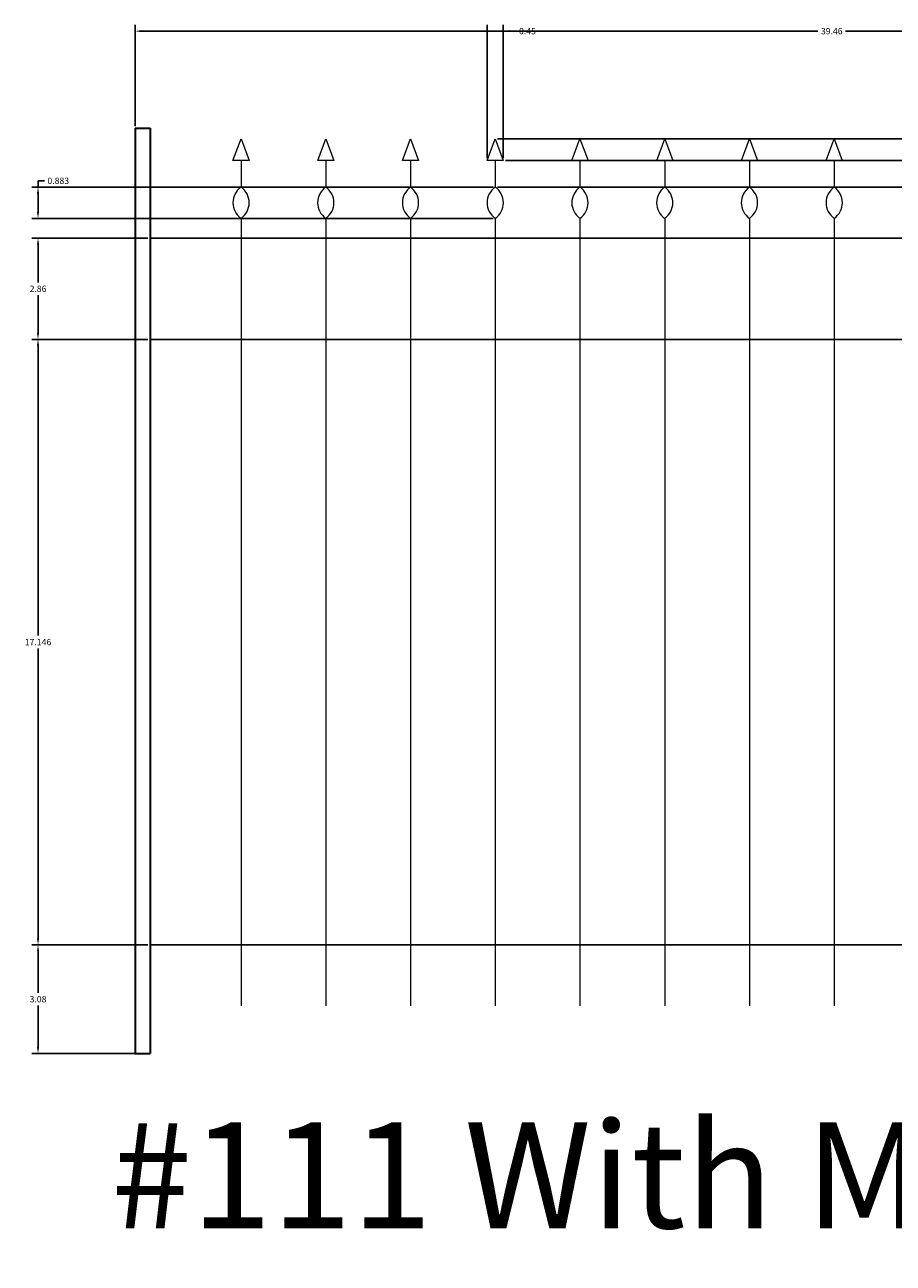
# Model space of a CAD drawing. Units: inches. Extents: x 756 to 915, y 488 to 695.
# Tile 24 of 25: x 863 to 888, y 660 to 695. Entities that reach past the tile are written whole.
import ezdxf

# ---------------------------------------------------------------- set-up
doc = ezdxf.new("R2010")
doc.units = ezdxf.units.IN
doc.header["$MEASUREMENT"] = 0
for name, color, linetype, lineweight in [('L-ANNO-TEXT', 7, 'Continuous', 25), ('L-FENC-PCKT', 7, 'Continuous', 18), ('L-FENC-POST', 7, 'Continuous', 35), ('L-FENC-RAIL', 7, 'Continuous', 25), ('M-DIMS', 2, 'Continuous', 18)]:
    doc.layers.add(name, color=color, linetype=linetype, lineweight=lineweight)
doc.styles.get("Standard").update_dxf_attribs({"font": 'arial.ttf'})
doc.dimstyles.get("Standard").update_dxf_attribs({"dimtxt": 0.18, "dimasz": 0.18, "dimexe": 0.18, "dimexo": 0.0625, "dimgap": 0.09, "dimtad": 0, "dimtih": 1, "dimtoh": 1, "dimdec": 0, "dimzin": 0, "dimdsep": 46, "dimlunit": 3, "dimtxsty": 'Standard', "dimcen": 0.09, "dimadec": 0, "dimazin": 0, "dimtfac": 1, "dimtdec": 0, "dimtofl": 0, "dimtmove": 0, "dimatfit": 3, "dimfxl": 1, "dimtolj": 1, "dimtzin": 0, "dimarcsym": 0})

# ---------------------------------------------------------------- blocks, each defined once
blk = doc.blocks.new('PICKET-MAJESTIC-EXTENDED')
for p, q in [((0.231, 23.946), (0.231, 23.188)), ((0.231, 22.305), (0.231, 0))]:
    blk.add_line(p, q)
blk.add_lwpolyline([(0.231, 23.946), (0.003, 23.946), (0.231, 24.558), (0.458, 23.946)], close=True)
blk.add_lwpolyline([(0.231, 22.305, 0.522719), (0.231, 23.188, 0.522719)], format="xyb", close=True)
blk = doc.blocks.new('FENCE-POST-LEFT')
for p, q in [((0, 26.207), (0, 0)), ((0, 26.207), (0.426, 26.207)), ((0.426, 26.207), (0.426, 0)), ((0.426, 26.207), (0.426, 0)), ((0, 0), (0.426, 0))]:
    blk.add_line(p, q)
blk = doc.blocks.new('*D23')
at = {"layer": 'Defpoints', "color": 0, "transparency": 16777216}
for p in [(905.684, 694.703), (866.226, 691.953), (905.684, 691.953)]:
    blk.add_point(p, dxfattribs=at)
at = {"layer": 'M-DIMS', "color": 0, "lineweight": -2, "transparency": 16777216}
for p, q in [((866.226, 692.015), (866.226, 694.883)), ((905.684, 692.015), (905.684, 694.883)), ((866.406, 694.703), (885.561, 694.703)), ((905.504, 694.703), (886.348, 694.703))]:
    blk.add_line(p, q, dxfattribs=at)
at = {"layer": 'M-DIMS', "color": 0, "transparency": 16777216}
for points in [[(866.406, 694.733), (866.406, 694.673), (866.226, 694.703)], [(905.504, 694.733), (905.504, 694.673), (905.684, 694.703)]]:
    blk.add_solid(points, dxfattribs=at)
at = {"layer": 'M-DIMS', "color": 0, "transparency": 16777216, "insert": (885.955, 694.703), "char_height": 0.18, "attachment_point": 5}
blk.add_mtext('\\A1;39.46', dxfattribs=at)
blk = doc.blocks.new('*D25')
at = {"layer": 'Defpoints', "color": 0, "transparency": 16777216}
for p in [(863.476, 685.974), (866.652, 685.974), (866.652, 668.828)]:
    blk.add_point(p, dxfattribs=at)
at = {"layer": 'M-DIMS', "color": 0, "lineweight": -2, "transparency": 16777216}
for p, q in [((866.59, 685.974), (863.296, 685.974)), ((863.476, 685.794), (863.476, 677.583)), ((863.476, 669.008), (863.476, 677.219)), ((866.59, 668.828), (863.296, 668.828))]:
    blk.add_line(p, q, dxfattribs=at)
at = {"layer": 'M-DIMS', "color": 0, "transparency": 16777216}
for points in [[(863.446, 685.794), (863.506, 685.794), (863.476, 685.974)], [(863.446, 669.008), (863.506, 669.008), (863.476, 668.828)]]:
    blk.add_solid(points, dxfattribs=at)
at = {"layer": 'M-DIMS', "color": 0, "transparency": 16777216, "insert": (863.476, 677.401), "char_height": 0.18, "attachment_point": 5}
blk.add_mtext('\\A1;17.146', dxfattribs=at)
blk = doc.blocks.new('*D26')
at = {"layer": 'Defpoints', "color": 0, "transparency": 16777216}
for p in [(863.476, 688.838), (866.652, 688.838), (866.652, 685.974)]:
    blk.add_point(p, dxfattribs=at)
at = {"layer": 'M-DIMS', "color": 0, "lineweight": -2, "transparency": 16777216}
for p, q in [((866.59, 688.838), (863.296, 688.838)), ((863.476, 688.658), (863.476, 687.588)), ((863.476, 686.154), (863.476, 687.224)), ((866.59, 685.974), (863.296, 685.974))]:
    blk.add_line(p, q, dxfattribs=at)
at = {"layer": 'M-DIMS', "color": 0, "transparency": 16777216}
for points in [[(863.446, 688.658), (863.506, 688.658), (863.476, 688.838)], [(863.446, 686.154), (863.506, 686.154), (863.476, 685.974)]]:
    blk.add_solid(points, dxfattribs=at)
at = {"layer": 'M-DIMS', "color": 0, "transparency": 16777216, "insert": (863.476, 687.406), "char_height": 0.18, "attachment_point": 5}
blk.add_mtext('\\A1;2.86', dxfattribs=at)
blk = doc.blocks.new('*D27')
at = {"layer": 'Defpoints', "color": 0, "transparency": 16777216}
for p in [(863.476, 668.828), (866.652, 668.828), (866.652, 665.746)]:
    blk.add_point(p, dxfattribs=at)
at = {"layer": 'M-DIMS', "color": 0, "lineweight": -2, "transparency": 16777216}
for p, q in [((866.59, 668.828), (863.296, 668.828)), ((863.476, 668.648), (863.476, 667.469)), ((863.476, 665.926), (863.476, 667.105)), ((866.59, 665.746), (863.296, 665.746))]:
    blk.add_line(p, q, dxfattribs=at)
at = {"layer": 'M-DIMS', "color": 0, "transparency": 16777216}
for points in [[(863.446, 668.648), (863.506, 668.648), (863.476, 668.828)], [(863.446, 665.926), (863.506, 665.926), (863.476, 665.746)]]:
    blk.add_solid(points, dxfattribs=at)
at = {"layer": 'M-DIMS', "color": 0, "transparency": 16777216, "insert": (863.476, 667.287), "char_height": 0.18, "attachment_point": 5}
blk.add_mtext('\\A1;3.08', dxfattribs=at)
blk = doc.blocks.new('*D28')
at = {"layer": 'Defpoints', "color": 0, "transparency": 16777216}
for p in [(876.652, 694.703), (876.197, 691.042), (876.652, 691.042)]:
    blk.add_point(p, dxfattribs=at)
at = {"layer": 'M-DIMS', "color": 0, "lineweight": -2, "transparency": 16777216}
for p, q in [((876.197, 691.104), (876.197, 694.883)), ((876.652, 691.104), (876.652, 694.883)), ((876.017, 694.703), (875.837, 694.703)), ((876.832, 694.703), (877.012, 694.703))]:
    blk.add_line(p, q, dxfattribs=at)
at = {"layer": 'M-DIMS', "color": 0, "transparency": 16777216}
for points in [[(876.017, 694.733), (876.017, 694.673), (876.197, 694.703)], [(876.832, 694.733), (876.832, 694.673), (876.652, 694.703)]]:
    blk.add_solid(points, dxfattribs=at)
at = {"layer": 'M-DIMS', "color": 0, "transparency": 16777216, "insert": (877.336, 694.703), "char_height": 0.18, "attachment_point": 5}
blk.add_mtext('\\A1;0.45', dxfattribs=at)
blk = doc.blocks.new('*D29')
at = {"layer": 'Defpoints', "color": 0, "transparency": 16777216}
for p in [(876.424, 691.654), (908.434, 691.654), (876.652, 691.042)]:
    blk.add_point(p, dxfattribs=at)
at = {"layer": 'M-DIMS', "color": 0, "lineweight": -2, "transparency": 16777216}
for p, q in [((876.487, 691.654), (908.614, 691.654)), ((908.434, 691.654), (908.434, 691.834)), ((908.434, 691.834), (908.614, 691.834)), ((908.434, 691.222), (908.434, 691.474)), ((876.714, 691.042), (908.614, 691.042))]:
    blk.add_line(p, q, dxfattribs=at)
at = {"layer": 'M-DIMS', "color": 0, "transparency": 16777216}
for points in [[(908.404, 691.474), (908.464, 691.474), (908.434, 691.654)], [(908.404, 691.222), (908.464, 691.222), (908.434, 691.042)]]:
    blk.add_solid(points, dxfattribs=at)
at = {"layer": 'M-DIMS', "color": 0, "transparency": 16777216, "insert": (909.006, 691.834), "char_height": 0.18, "attachment_point": 5}
blk.add_mtext('\\A1;0.612', dxfattribs=at)
blk = doc.blocks.new('*D30')
at = {"layer": 'Defpoints', "color": 0, "transparency": 16777216}
for p in [(876.652, 691.042), (908.434, 691.042), (876.424, 690.284)]:
    blk.add_point(p, dxfattribs=at)
at = {"layer": 'M-DIMS', "color": 0, "lineweight": -2, "transparency": 16777216}
for p, q in [((876.714, 691.042), (908.614, 691.042)), ((908.434, 691.042), (908.434, 691.222)), ((908.434, 691.222), (908.614, 691.222)), ((908.434, 690.464), (908.434, 690.862)), ((876.487, 690.284), (908.614, 690.284))]:
    blk.add_line(p, q, dxfattribs=at)
at = {"layer": 'M-DIMS', "color": 0, "transparency": 16777216}
for points in [[(908.404, 690.862), (908.464, 690.862), (908.434, 691.042)], [(908.404, 690.464), (908.464, 690.464), (908.434, 690.284)]]:
    blk.add_solid(points, dxfattribs=at)
at = {"layer": 'M-DIMS', "color": 0, "transparency": 16777216, "insert": (908.937, 691.222), "char_height": 0.18, "attachment_point": 5}
blk.add_mtext('\\A1;0.76', dxfattribs=at)
blk = doc.blocks.new('*D31')
at = {"layer": 'Defpoints', "color": 0, "transparency": 16777216}
for p in [(863.476, 690.284), (876.424, 690.284), (876.424, 689.401)]:
    blk.add_point(p, dxfattribs=at)
at = {"layer": 'M-DIMS', "color": 0, "lineweight": -2, "transparency": 16777216}
for p, q in [((876.362, 690.284), (863.296, 690.284)), ((863.476, 690.284), (863.476, 690.464)), ((863.476, 690.464), (863.656, 690.464)), ((863.476, 689.581), (863.476, 690.104)), ((876.362, 689.401), (863.296, 689.401))]:
    blk.add_line(p, q, dxfattribs=at)
at = {"layer": 'M-DIMS', "color": 0, "transparency": 16777216}
for points in [[(863.446, 690.104), (863.506, 690.104), (863.476, 690.284)], [(863.446, 689.581), (863.506, 689.581), (863.476, 689.401)]]:
    blk.add_solid(points, dxfattribs=at)
at = {"layer": 'M-DIMS', "color": 0, "transparency": 16777216, "insert": (864.049, 690.464), "char_height": 0.18, "attachment_point": 5}
blk.add_mtext('\\A1;0.883', dxfattribs=at)

msp = doc.modelspace()

# ---------------------------------------------------------------- linework, layer by layer
at = {"layer": 'L-FENC-RAIL'}
for p, q in [((866.6522, 688.8379), (905.257, 688.8379)), ((866.6522, 685.9735), (905.257, 685.9735)), ((866.6522, 668.8277), (905.257, 668.8277))]:
    msp.add_line(p, q, dxfattribs=at)

# ---------------------------------------------------------------- block references
at = {"layer": 'L-FENC-PCKT'}
for p in [(868.994, 667.096), (871.3939, 667.096), (873.7938, 667.096), (876.1937, 667.096), (878.5936, 667.096), (880.9936, 667.096), (883.3935, 667.096), (885.7934, 667.096)]:
    msp.add_blockref('PICKET-MAJESTIC-EXTENDED', p, dxfattribs=at)
at = {"layer": 'L-FENC-POST'}
msp.add_blockref('FENCE-POST-LEFT', (866.2259, 665.746), dxfattribs=at)

# ---------------------------------------------------------------- texts
at = {"layer": 'L-ANNO-TEXT'}
msp.add_text('#111 With Mejestic Finais', height=3, dxfattribs=at).set_placement((865.5471, 660.7997))

# ---------------------------------------------------------------- dimensions: what is measured, and where the dimension line sits
at = {"layer": 'M-DIMS'}
for base, p1, p2, picture, middle in [((905.6837, 694.7029), (866.2255, 691.9529), (905.6837, 691.9529), '*D23', (885.9546, 694.7029)), ((876.6517, 694.7029), (876.1971, 691.0419), (876.6517, 691.0419), '*D28', (877.3361, 694.7029))]:
    dim = msp.add_linear_dim(base=base, p1=p1, p2=p2, dimstyle='Standard', override={"dimdec": 2, "dimlfac": 1, "dimrnd": 0, "dimzin": 0, "dimdsep": 46, "dimlunit": 2}, dxfattribs=at)
    dim.commit()
    dim.dimension.update_dxf_attribs({"geometry": picture, "text_midpoint": middle})
for base, p1, p2, override, picture, middle in [((908.4337, 691.6538), (876.6517, 691.0419), (876.4244, 691.6538), {"dimdec": 3, "dimlfac": 1, "dimrnd": 0, "dimzin": 0, "dimdsep": 46, "dimlunit": 2}, '*D29', (909.0065, 691.8338)), ((908.4337, 691.0419), (876.4244, 690.2836), (876.6517, 691.0419), {"dimdec": 2, "dimlfac": 1, "dimrnd": 0, "dimzin": 0, "dimdsep": 46, "dimlunit": 2}, '*D30', (908.9374, 691.2219)), ((863.4755, 690.2836), (876.4244, 689.4007), (876.4244, 690.2836), {"dimdec": 3, "dimlfac": 1, "dimrnd": 0, "dimzin": 0, "dimdsep": 46, "dimlunit": 2}, '*D31', (864.0492, 690.4636)), ((863.4755, 688.8379), (866.6522, 685.9735), (866.6522, 688.8379), {"dimdec": 2, "dimlfac": 1, "dimrnd": 0, "dimzin": 0, "dimdsep": 46, "dimlunit": 2}, '*D26', (863.4755, 687.4057)), ((863.4755, 685.9735), (866.6522, 668.8277), (866.6522, 685.9735), {"dimdec": 3, "dimlfac": 1, "dimrnd": 0, "dimzin": 0, "dimdsep": 46, "dimlunit": 2}, '*D25', (863.4755, 677.4006)), ((863.4755, 668.8277), (866.6522, 665.7461), (866.6522, 668.8277), {"dimdec": 2, "dimlfac": 1, "dimrnd": 0, "dimzin": 0, "dimdsep": 46, "dimlunit": 2}, '*D27', (863.4755, 667.2869))]:
    dim = msp.add_linear_dim(base=base, p1=p1, p2=p2, angle=90, dimstyle='Standard', override=override, dxfattribs=at)
    dim.commit()
    dim.dimension.update_dxf_attribs({"geometry": picture, "text_midpoint": middle})

doc.saveas('drawing.dxf')
